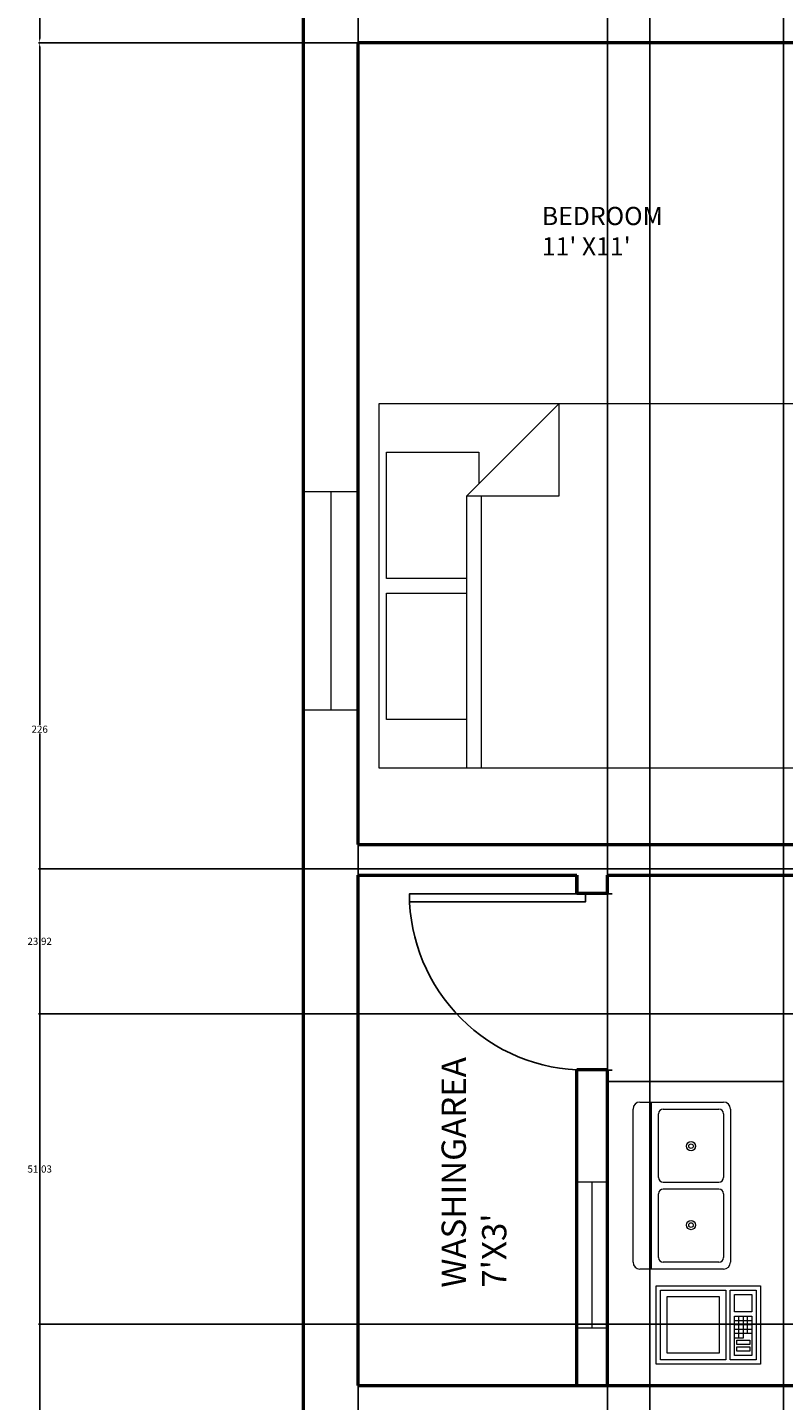
# Model space of a CAD drawing. Units: inches. Extents: x 3506 to 3958, y 1553 to 2506.
# Tile 9 of 16: x 3506 to 3631, y 2003 to 2229. Entities that reach past the tile are written whole.
import ezdxf

# ---------------------------------------------------------------- set-up
doc = ezdxf.new("R2010")
doc.units = ezdxf.units.IN
doc.header["$MEASUREMENT"] = 0
for name, color, linetype, lineweight in [('A-ANNO-DIMS', 2, 'Continuous', 18), ('A-AREA-IDEN', 7, 'Continuous', 18), ('A-FLOR-CASE', 7, 'Continuous', 25), ('A-WALL', 7, 'Continuous', 50), ('doors', 40, 'Continuous', 25), ('furniture', 120, 'Continuous', 18), ('kitchen', 181, 'Continuous', 18), ('window', 30, 'Continuous', 20)]:
    doc.layers.add(name, color=color, linetype=linetype, lineweight=lineweight)
doc.layers.add('A-WALL-PATT', color=251, linetype='Continuous', lineweight=13, true_color=0x636466)
doc.styles.get("Standard").update_dxf_attribs({"font": 'arial.ttf'})
doc.dimstyles.get("Standard").update_dxf_attribs({"dimtxt": 1.18, "dimasz": 0.68, "dimexe": 0.18, "dimexo": 0.0625, "dimgap": 0.09, "dimtad": 0, "dimtih": 1, "dimtoh": 1, "dimdec": 1, "dimzin": 0, "dimdsep": 46, "dimlunit": 3, "dimtxsty": 'Standard', "dimcen": 0.09, "dimadec": 0, "dimazin": 0, "dimtfac": 1, "dimtdec": 1, "dimtofl": 0, "dimtmove": 0, "dimatfit": 3, "dimfxl": 1, "dimtolj": 1, "dimtzin": 0, "dimarcsym": 0})

# ---------------------------------------------------------------- blocks, each defined once
blk = doc.blocks.new('*U12')
for p, q in [((0, 0), (0, 6)), ((40, 0), (40, 6))]:
    blk.add_line(p, q)
blk.add_lwpolyline([(0, 0), (0, -40), (1.75, -40), (1.75, 0)], close=True)
blk.add_arc((0, 0), 40, 270, 0)
blk = doc.blocks.new('Bed - Queen')
for p, q in [((0, -80.00003), (0, 0)), ((0, 0), (59.99999, 0)), ((59.99999, 0), (59.99999, -80.00003)), ((7.99999, -1.2), (28.79998, -1.2)), ((7.99999, -14.4), (7.99999, -1.2)), ((28.79998, -1.2), (28.79998, -14.4)), ((31.19999, -1.2), (51.99999, -1.2)), ((31.19999, -14.4), (31.19999, -1.2)), ((51.99999, -1.2), (51.99999, -16.4)), ((0, -14.4), (44.8, -14.4)), ((59.99999, -29.6), (44.8, -14.4)), ((44.8, -14.4), (44.8, -29.6)), ((44.8, -16.8), (0, -16.8)), ((51.99999, -16.4), (46.79936, -16.4)), ((44.8, -29.6), (59.99999, -29.6)), ((59.99999, -80.00003), (0, -80.00003))]:
    blk.add_line(p, q)
blk = doc.blocks.new('Microwave')
for p, q in [((18, 10), (22, 10)), ((19, 7), (19, 11)), ((20, 11), (20, 7)), ((21, 7), (21, 11)), ((22, 9), (18, 9)), ((18, 8), (22, 8)), ((22, 7), (18, 7)), ((19, 6), (19, 7)), ((20, 7), (20, 6)), ((20, 6), (18, 6))]:
    blk.add_line(p, q)
for points in [[(0, 0), (0, 18), (24, 18), (24, 0)], [(1, 1), (1, 17), (16, 17), (16, 1)], [(17, 1), (17, 17), (23, 17), (23, 1)], [(18, 12), (18, 16), (22, 16), (22, 12)], [(2.5, 2.5), (2.5, 15.5), (14.5, 15.5), (14.5, 2.5)], [(18, 2), (18, 11), (22, 11), (22, 2)], [(18.5, 4.5), (18.5, 5.5), (21.5, 5.5), (21.5, 4.5)], [(18.5, 3), (18.5, 4), (21.5, 4), (21.5, 3)]]:
    blk.add_lwpolyline(points, close=True)
blk = doc.blocks.new('Sink-double - 36 in top')
for p, q in [((-18, -4), (18, -4)), ((-0.75, -18.5), (-0.75, -6.5)), ((0.75, -6.5), (0.75, -18.5))]:
    blk.add_line(p, q)
for points in [[(-16.5, 0), (16.5, 0)], [(-18, -19.5), (-18, -1.5)], [(18, -1.5), (18, -19.5)], [(-15.5, -5.5), (-1.75, -5.5)], [(1.75, -5.5), (15.5, -5.5)], [(-16.5, -18.5), (-16.5, -6.5)], [(16.5, -6.5), (16.5, -18.5)], [(-1.75, -19.5), (-15.5, -19.5)], [(15.5, -19.5), (1.75, -19.5)], [(16.5, -21), (-16.5, -21)]]:
    blk.add_lwpolyline(points)
for centre, radius in [((-8.5, -12.5), 1), ((8.5, -12.5), 1), ((-8.5, -12.5), 0.5), ((8.5, -12.5), 0.5)]:
    blk.add_circle(centre, radius)
for centre, radius, start, end in [((-16.5, -1.5), 1.5, 90, 180), ((16.5, -1.5), 1.5, 0, 90), ((-15.5, -6.5), 1, 90, 180), ((-1.75, -6.5), 1, 0, 90), ((1.75, -6.5), 1, 90, 180), ((15.5, -6.5), 1, 0, 90), ((-16.5, -19.5), 1.5, 180, 270), ((-15.5, -18.5), 1, 180, 270), ((-1.75, -18.5), 1, 270, 0), ((1.75, -18.5), 1, 180, 270), ((15.5, -18.5), 1, 270, 0), ((16.5, -19.5), 1.5, 270, 0)]:
    blk.add_arc(centre, radius, start, end)
blk = doc.blocks.new('WIN-24IN-5IN-PARTITION')
for p, q in [((5, 24), (0, 24)), ((0, 24), (0, 0)), ((2.5, 0), (2.5, 24)), ((5, 0), (5, 24)), ((0, 0), (5, 0)), ((0, 0), (2.5, 0))]:
    blk.add_line(p, q)
blk = doc.blocks.new('*D43')
at = {"layer": 'A-ANNO-DIMS', "color": 0, "lineweight": -2, "transparency": 16777216}
for p, q in [((3560.67, 2226.39), (3508.1, 2226.39)), ((3508.28, 2225.71), (3508.28, 2114.09)), ((3508.28, 2001.07), (3508.28, 2112.7)), ((3560.67, 2000.39), (3508.1, 2000.39))]:
    blk.add_line(p, q, dxfattribs=at)
at = {"layer": 'A-ANNO-DIMS', "color": 0, "transparency": 16777216}
for points in [[(3508.17, 2225.71), (3508.39, 2225.71), (3508.28, 2226.39)], [(3508.17, 2001.07), (3508.39, 2001.07), (3508.28, 2000.39)]]:
    blk.add_solid(points, dxfattribs=at)
at = {"layer": 'Defpoints', "color": 0, "transparency": 16777216}
for p in [(3508.28, 2226.39), (3560.73, 2226.39), (3560.73, 2000.39)]:
    blk.add_point(p, dxfattribs=at)
at = {"layer": 'A-ANNO-DIMS', "color": 0, "transparency": 16777216, "insert": (3508.28, 2113.39), "char_height": 1.18, "attachment_point": 5}
blk.add_mtext('\\A1;226', dxfattribs=at)
blk = doc.blocks.new('*D44')
at = {"layer": 'A-ANNO-DIMS', "color": 0, "lineweight": -2, "transparency": 16777216}
for p, q in [((3911.67, 2461.39), (3508.1, 2461.39)), ((3508.28, 2460.71), (3508.28, 2344.59)), ((3508.28, 2227.07), (3508.28, 2343.2)), ((3560.67, 2226.39), (3508.1, 2226.39))]:
    blk.add_line(p, q, dxfattribs=at)
at = {"layer": 'A-ANNO-DIMS', "color": 0, "transparency": 16777216}
for points in [[(3508.17, 2460.71), (3508.39, 2460.71), (3508.28, 2461.39)], [(3508.17, 2227.07), (3508.39, 2227.07), (3508.28, 2226.39)]]:
    blk.add_solid(points, dxfattribs=at)
at = {"layer": 'Defpoints', "color": 0, "transparency": 16777216}
for p in [(3508.28, 2461.39), (3911.73, 2461.39), (3560.73, 2226.39)]:
    blk.add_point(p, dxfattribs=at)
at = {"layer": 'A-ANNO-DIMS', "color": 0, "transparency": 16777216, "insert": (3508.28, 2343.89), "char_height": 1.18, "attachment_point": 5}
blk.add_mtext('\\A1;235', dxfattribs=at)
blk = doc.blocks.new('*D50')
at = {"layer": 'A-ANNO-DIMS', "color": 0, "lineweight": -2, "transparency": 16777216}
for p, q in [((3608.73, 1606.46), (3608.73, 2505.02)), ((3609.41, 2504.84), (3672.39, 2504.84)), ((3738.05, 2504.84), (3675.07, 2504.84)), ((3738.73, 1606.46), (3738.73, 2505.02))]:
    blk.add_line(p, q, dxfattribs=at)
at = {"layer": 'A-ANNO-DIMS', "color": 0, "transparency": 16777216}
for points in [[(3609.41, 2504.96), (3609.41, 2504.73), (3608.73, 2504.84)], [(3738.05, 2504.96), (3738.05, 2504.73), (3738.73, 2504.84)]]:
    blk.add_solid(points, dxfattribs=at)
at = {"layer": 'Defpoints', "color": 0, "transparency": 16777216}
for p in [(3738.73, 2504.84), (3608.73, 1606.39), (3738.73, 1606.39)]:
    blk.add_point(p, dxfattribs=at)
at = {"layer": 'A-ANNO-DIMS', "color": 0, "transparency": 16777216, "insert": (3673.73, 2504.84), "char_height": 1.18, "attachment_point": 5}
blk.add_mtext('\\A1;130', dxfattribs=at)
blk = doc.blocks.new('*D52')
at = {"layer": 'A-ANNO-DIMS', "color": 0, "lineweight": -2, "transparency": 16777216}
for p, q in [((3560.73, 1606.46), (3560.73, 2505.02)), ((3561.41, 2504.84), (3583.77, 2504.84)), ((3608.05, 2504.84), (3585.69, 2504.84)), ((3608.73, 1606.46), (3608.73, 2505.02))]:
    blk.add_line(p, q, dxfattribs=at)
at = {"layer": 'A-ANNO-DIMS', "color": 0, "transparency": 16777216}
for points in [[(3561.41, 2504.96), (3561.41, 2504.73), (3560.73, 2504.84)], [(3608.05, 2504.96), (3608.05, 2504.73), (3608.73, 2504.84)]]:
    blk.add_solid(points, dxfattribs=at)
at = {"layer": 'Defpoints', "color": 0, "transparency": 16777216}
for p in [(3608.73, 2504.84), (3560.73, 1606.39), (3608.73, 1606.39)]:
    blk.add_point(p, dxfattribs=at)
at = {"layer": 'A-ANNO-DIMS', "color": 0, "transparency": 16777216, "insert": (3584.73, 2504.84), "char_height": 1.18, "attachment_point": 5}
blk.add_mtext('\\A1;48', dxfattribs=at)
blk = doc.blocks.new('*D60')
at = {"layer": 'A-ANNO-DIMS', "color": 0, "lineweight": -2, "transparency": 16777216}
for p, q in [((3860.67, 2066.52), (3508.1, 2066.52)), ((3508.28, 2065.84), (3508.28, 2041.7)), ((3508.28, 2016.17), (3508.28, 2040.31)), ((3860.67, 2015.49), (3508.1, 2015.49))]:
    blk.add_line(p, q, dxfattribs=at)
at = {"layer": 'A-ANNO-DIMS', "color": 0, "transparency": 16777216}
for points in [[(3508.17, 2065.84), (3508.39, 2065.84), (3508.28, 2066.52)], [(3508.17, 2016.17), (3508.39, 2016.17), (3508.28, 2015.49)]]:
    blk.add_solid(points, dxfattribs=at)
at = {"layer": 'Defpoints', "color": 0, "transparency": 16777216}
for p in [(3860.73, 2066.52), (3508.28, 2015.49), (3860.73, 2015.49)]:
    blk.add_point(p, dxfattribs=at)
at = {"layer": 'A-ANNO-DIMS', "color": 0, "transparency": 16777216, "insert": (3508.28, 2041), "char_height": 1.18, "attachment_point": 5}
blk.add_mtext('\\A1;51.03', dxfattribs=at)
blk = doc.blocks.new('*D61')
at = {"layer": 'A-ANNO-DIMS', "color": 0, "lineweight": -2, "transparency": 16777216}
for p, q in [((3860.67, 2090.43), (3508.1, 2090.43)), ((3508.28, 2089.75), (3508.28, 2079.17)), ((3508.28, 2067.2), (3508.28, 2077.78)), ((3860.67, 2066.52), (3508.1, 2066.52))]:
    blk.add_line(p, q, dxfattribs=at)
at = {"layer": 'A-ANNO-DIMS', "color": 0, "transparency": 16777216}
for points in [[(3508.17, 2089.75), (3508.39, 2089.75), (3508.28, 2090.43)], [(3508.17, 2067.2), (3508.39, 2067.2), (3508.28, 2066.52)]]:
    blk.add_solid(points, dxfattribs=at)
at = {"layer": 'Defpoints', "color": 0, "transparency": 16777216}
for p in [(3860.73, 2090.43), (3508.28, 2066.52), (3860.73, 2066.52)]:
    blk.add_point(p, dxfattribs=at)
at = {"layer": 'A-ANNO-DIMS', "color": 0, "transparency": 16777216, "insert": (3508.28, 2078.48), "char_height": 1.18, "attachment_point": 5}
blk.add_mtext('\\A1;23.92', dxfattribs=at)
blk = doc.blocks.new('*D68')
at = {"layer": 'A-ANNO-DIMS', "color": 0, "lineweight": -2, "transparency": 16777216}
for p, q in [((3630.73, 2260.33), (3630.73, 1553.76)), ((3601.73, 2231.33), (3601.73, 1553.76)), ((3602.41, 1553.94), (3615.28, 1553.94)), ((3630.05, 1553.94), (3617.18, 1553.94))]:
    blk.add_line(p, q, dxfattribs=at)
at = {"layer": 'A-ANNO-DIMS', "color": 0, "transparency": 16777216}
for points in [[(3602.41, 1554.06), (3602.41, 1553.83), (3601.73, 1553.94)], [(3630.05, 1554.06), (3630.05, 1553.83), (3630.73, 1553.94)]]:
    blk.add_solid(points, dxfattribs=at)
at = {"layer": 'Defpoints', "color": 0, "transparency": 16777216}
for p in [(3630.73, 2260.39), (3601.73, 2231.39), (3630.73, 1553.94)]:
    blk.add_point(p, dxfattribs=at)
at = {"layer": 'A-ANNO-DIMS', "color": 0, "transparency": 16777216, "insert": (3616.23, 1553.94), "char_height": 1.18, "attachment_point": 5}
blk.add_mtext('\\A1;29', dxfattribs=at)

msp = doc.modelspace()

# ---------------------------------------------------------------- hatches: boundary and pattern name
at = {"layer": 'A-WALL-PATT'}
h = msp.add_hatch(dxfattribs=at)
h.set_pattern_fill('ANSI31', color=256)
h.paths.add_polyline_path([(3911.7302, 2461.3942), (3551.7302, 2461.3942), (3551.7302, 2152.516), (3560.7302, 2152.516), (3560.7302, 2116.516), (3551.7302, 2116.516), (3551.7302, 1920.5711), (3556.2302, 1920.5711), (3560.7302, 1920.5711), (3560.7302, 2000.3942), (3692.7302, 2000.3942), (3692.7302, 1997.3942), (3697.7302, 1997.3942), (3697.7302, 2000.3942), (3771.7302, 2000.3942), (3771.7302, 1997.3942), (3776.7302, 1997.3942), (3776.7302, 1997.7206), (3778.5802, 1997.7206), (3807.5802, 1997.7206), (3807.5802, 1996.4519), (3778.5802, 1996.4519), (3778.5802, 1997.7206), (3776.7302, 1997.7206), (3776.7302, 1997.3942), (3771.7302, 1997.3942), (3771.7302, 2000.3942), (3697.7302, 2000.3942), (3697.7302, 1997.3942), (3692.7302, 1997.3942), (3689.8302, 1997.3942), (3689.8302, 1995.8192), (3653.8302, 1995.8192), (3653.8302, 1997.3942), (3689.8302, 1997.3942), (3692.7302, 1997.3942), (3692.7302, 2000.3942), (3560.7302, 2000.3942), (3560.7302, 1920.5711), (3551.7302, 1920.5711), (3551.7302, 1884.5711), (3551.7302, 1597.3942), (3911.7302, 1597.3942)], flags=17)
h.paths.add_polyline_path([(3596.7302, 2005.3942), (3596.7302, 2057.3035, -0.38730371), (3569.1778, 2085), (3569.15, 2085), (3569.15, 2086.2688), (3598.15, 2086.2688), (3598.15, 2085), (3569.1778, 2085, 0.38730371), (3596.7302, 2057.3035), (3596.7302, 2057.3942), (3601.7302, 2057.3942), (3601.7302, 2055.3942), (3630.7302, 2055.3942), (3630.7302, 2034.3942), (3694.7302, 2034.3942), (3694.7302, 2053.3942), (3699.7302, 2053.3942), (3699.7302, 2005.3942), (3860.7302, 2005.3942), (3860.7302, 2173.3942), (3771.7302, 2173.3942), (3771.7302, 2194.3942), (3776.7302, 2194.3942), (3776.7302, 2178.3942), (3860.7302, 2178.3942), (3860.7302, 2231.3942), (3601.7302, 2231.3942), (3601.7302, 2241.426), (3596.7302, 2241.426), (3596.7302, 2231.3942), (3560.7302, 2231.3942), (3560.7302, 2315.3942), (3596.7302, 2315.3942), (3596.7302, 2312.3942), (3601.7302, 2312.3942), (3601.7302, 2315.3942), (3697.7302, 2315.3942), (3697.7302, 2413.3942), (3692.7302, 2413.3942), (3692.7302, 2320.3942), (3560.7302, 2320.3942), (3560.7302, 2452.3942), (3692.7302, 2452.3942), (3692.7302, 2449.3942), (3697.7302, 2449.3942), (3697.7302, 2452.3942), (3771.7302, 2452.3942), (3771.7302, 2449.3942), (3776.7302, 2449.3942), (3776.7302, 2452.3942), (3860.7302, 2452.3942), (3860.7302, 2437.2075), (3865.2302, 2437.2075), (3865.2302, 2413.2075), (3860.7302, 2413.2075), (3860.7302, 2367.6976), (3865.2302, 2367.6976), (3869.7302, 2367.6976), (3869.7302, 2319.6976), (3860.7302, 2319.6976), (3860.7302, 2211.6248), (3869.7302, 2211.6248), (3869.7302, 2187.6248), (3860.7302, 2187.6248), (3860.7302, 2138.4346), (3865.2302, 2138.4346), (3869.7302, 2138.4346), (3869.7302, 2090.4346), (3860.7302, 2090.4346), (3860.7302, 1985.8449), (3869.7302, 1985.8449), (3869.7302, 1961.8449), (3860.7302, 1961.8449), (3860.7302, 1897.0756), (3865.2302, 1897.0756), (3869.7302, 1897.0756), (3869.7302, 1849.0756), (3860.7302, 1849.0756), (3860.7302, 1847.8112), (3860.7302, 1779.3942), (3596.7302, 1779.3942), (3596.7302, 1831.3942), (3601.7302, 1831.3942), (3601.7302, 1828.3942), (3630.7302, 1828.3942), (3630.7302, 1808.3942), (3691.7302, 1808.3942), (3691.7302, 1815.3942), (3696.7302, 1815.3942), (3696.7302, 1779.3942), (3860.7302, 1779.3942), (3860.7302, 1947.3942), (3771.7302, 1947.3942), (3771.7302, 1968.3942), (3776.7302, 1968.3942), (3776.7302, 1952.3942), (3860.7302, 1952.3942), (3860.7302, 2005.3942)], flags=0)
h.paths.add_polyline_path([(3596.7302, 2038.8546), (3601.7302, 2038.8546), (3601.7302, 2014.8546), (3596.7302, 2014.8546)], flags=0)
h.paths.add_polyline_path([(3564.1688, 2107), (3564.1688, 2167), (3644.1688, 2167), (3644.1688, 2107)], flags=0)
h.paths.add_polyline_path([(3607.0972, 2052.0208), (3620.8472, 2052.0208, -0.41421356), (3621.9931, 2050.875), (3621.9931, 2025.6667, -0.41421356), (3620.8472, 2024.5208), (3607.0972, 2024.5208, -0.41421356), (3605.9514, 2025.6667), (3605.9514, 2050.875, -0.41421356)], flags=0)
h.paths.add_polyline_path([(3578.5688, 2115), (3565.3688, 2115), (3565.3688, 2135.8), (3578.5688, 2135.8), (3578.5688, 2138.2), (3565.3688, 2138.2), (3565.3688, 2159), (3580.5688, 2159), (3580.5688, 2153.8), (3593.7688, 2167), (3593.7688, 2151.8), (3578.5688, 2151.8)], flags=0)
h.paths.add_polyline_path([(3610.9167, 2050.875), (3620.0833, 2050.875, -0.41421356), (3620.8472, 2050.1111), (3620.8472, 2039.6076, -0.41421356), (3620.0833, 2038.8438), (3610.9167, 2038.8438, -0.41421356), (3610.1528, 2039.6076), (3610.1528, 2050.1111, -0.41421356)], flags=0)
h.paths.add_polyline_path([(3610.9167, 2037.6979), (3620.0833, 2037.6979, -0.41421356), (3620.8472, 2036.934), (3620.8472, 2026.4306, -0.41421356), (3620.0833, 2025.6667), (3610.9167, 2025.6667, -0.41421356), (3610.1528, 2026.4306), (3610.1528, 2036.934, -0.41421356)], flags=0)
h.paths.add_polyline_path([(3616.2639, 2044.7639, -1), (3614.7361, 2044.7639, -1)], flags=0)
h.paths.add_polyline_path([(3615.8819, 2044.7639, -1), (3615.1181, 2044.7639, -1)], flags=0)
h.paths.add_polyline_path([(3616.2639, 2031.7778, -1), (3614.7361, 2031.7778, -1)], flags=0)
h.paths.add_polyline_path([(3615.8819, 2031.7778, -1), (3615.1181, 2031.7778, -1)], flags=0)
h.paths.add_polyline_path([(3609.7539, 2021.7868), (3626.9586, 2021.7868), (3626.9586, 2008.8833), (3609.7539, 2008.8833)], flags=0)
h.paths.add_polyline_path([(3610.4708, 2021.07), (3621.2237, 2021.07), (3621.2237, 2009.6002), (3610.4708, 2009.6002)], flags=0)
h.paths.add_polyline_path([(3611.5461, 2019.9947), (3620.1484, 2019.9947), (3620.1484, 2010.6755), (3611.5461, 2010.6755)], flags=0)
h.paths.add_polyline_path([(3621.9405, 2021.07), (3626.2417, 2021.07), (3626.2417, 2009.6002), (3621.9405, 2009.6002)], flags=0)
h.paths.add_polyline_path([(3622.6574, 2020.3531), (3625.5248, 2020.3531), (3625.5248, 2017.4857), (3622.6574, 2017.4857)], flags=0)
h.paths.add_polyline_path([(3622.6574, 2016.7688), (3625.5248, 2016.7688), (3625.5248, 2010.317), (3622.6574, 2010.317)], flags=0)
h.paths.add_polyline_path([(3624.808, 2016.0519), (3624.808, 2013.9013), (3624.0911, 2013.9013), (3624.0911, 2013.1845), (3623.3743, 2013.1845), (3623.3743, 2013.9013), (3623.3743, 2016.0519)], flags=0)
h.paths.add_polyline_path([(3623.0158, 2012.8261), (3625.1664, 2012.8261), (3625.1664, 2012.1092), (3623.0158, 2012.1092)], flags=0)
h.paths.add_polyline_path([(3623.0158, 2011.7508), (3625.1664, 2011.7508), (3625.1664, 2011.0339), (3623.0158, 2011.0339)], flags=0)
h.paths.add_polyline_path([(3650.0591, 2031.8202), (3674.0368, 2031.8202), (3674.0368, 2012.638), (3669.2413, 2012.638), (3669.2413, 2011.8388), (3672.4383, 2011.8388), (3672.4383, 2011.0395), (3651.6576, 2011.0395), (3651.6576, 2011.8388), (3654.8546, 2011.8388), (3654.8546, 2012.638), (3650.0591, 2012.638)], flags=0)
h.paths.add_polyline_path([(3658.0517, 2024.6269, -1), (3651.6576, 2024.6269, -1)], flags=0)
h.paths.add_polyline_path([(3657.2524, 2024.6269, -1), (3652.4569, 2024.6269, -1)], flags=0)
h.paths.add_polyline_path([(3656.4532, 2024.6269, -1), (3653.2561, 2024.6269, -1)], flags=0)
h.paths.add_polyline_path([(3655.6539, 2024.6269, -1), (3654.0554, 2024.6269, -1)], flags=0)
h.paths.add_polyline_path([(3657.2524, 2017.4336, -1), (3652.4569, 2017.4336, -1)], flags=0)
h.paths.add_polyline_path([(3656.4532, 2017.4336, -1), (3653.2561, 2017.4336, -1)], flags=0)
h.paths.add_polyline_path([(3655.6539, 2017.4336, -1), (3654.0554, 2017.4336, -1)], flags=0)
h.paths.add_polyline_path([(3659.6502, 2027.8239), (3664.4457, 2027.8239), (3664.4457, 2015.0358), (3659.6502, 2015.0358)], flags=0)
h.paths.add_polyline_path([(3663.6465, 2027.0247), (3663.6465, 2015.8351), (3660.4494, 2015.8351), (3660.4494, 2027.0247)], flags=0)
h.paths.add_polyline_path([(3562.6688, 1945.5), (3642.6688, 1945.5), (3642.6688, 1885.5), (3562.6688, 1885.5)], flags=0)
h.paths.add_polyline_path([(3671.6391, 2024.6269, -1), (3666.8435, 2024.6269, -1)], flags=0)
h.paths.add_polyline_path([(3670.8398, 2024.6269, -1), (3667.6428, 2024.6269, -1)], flags=0)
h.paths.add_polyline_path([(3672.4383, 2017.4336, -1), (3666.0443, 2017.4336, -1)], flags=0)
h.paths.add_polyline_path([(3670.0405, 2024.6269, -1), (3668.442, 2024.6269, -1)], flags=0)
h.paths.add_polyline_path([(3671.6391, 2017.4336, -1), (3666.8435, 2017.4336, -1)], flags=0)
h.paths.add_polyline_path([(3670.8398, 2017.4336, -1), (3667.6428, 2017.4336, -1)], flags=0)
h.paths.add_polyline_path([(3592.2688, 1945.5), (3592.2688, 1930.3), (3577.0688, 1930.3), (3577.0688, 1893.5), (3563.8688, 1893.5), (3563.8688, 1914.3), (3577.0688, 1914.3), (3577.0688, 1916.7), (3563.8688, 1916.7), (3563.8688, 1937.5), (3579.0688, 1937.5), (3579.0688, 1932.3)], flags=0)
h.paths.add_polyline_path([(3670.0405, 2017.4336, -1), (3668.442, 2017.4336, -1)], flags=0)
h.paths.add_polyline_path([(3596.7302, 2283.3942), (3601.7302, 2283.3942), (3601.7302, 2265.426), (3599.2302, 2265.426), (3599.2302, 2241.426), (3596.7302, 2241.426), (3596.7302, 2265.426)], flags=0)
h.paths.add_polyline_path([(3596.7302, 1810.7006), (3601.7302, 1810.7006), (3601.7302, 1786.7006), (3596.7302, 1786.7006)], flags=0)
h.paths.add_polyline_path([(3560.7302, 1770.3942), (3738.7302, 1770.3942), (3738.7302, 1746.3942), (3738.7302, 1722.3942), (3748.7302, 1722.3942), (3748.7302, 1674.3942), (3560.7302, 1674.3942)], flags=0)
h.paths.add_polyline_path([(3728.7302, 1746.3942), (3728.7302, 1756.0642), (3738.7302, 1746.3942), (3728.7302, 1738.1582), (3728.7302, 1698.3942), (3591.2519, 1698.3942), (3591.2519, 1746.3942)], flags=0)
h.paths.add_polyline_path([(3771.7302, 2399.3942), (3771.7302, 2420.3942), (3776.7302, 2420.3942), (3776.7302, 2404.3942), (3776.7302, 2399.3942)], flags=0)
h.paths.add_polyline_path([(3911.7302, 2461.3942), (3551.7302, 2461.3942), (3551.7302, 2152.516), (3560.7302, 2152.516), (3560.7302, 2116.516), (3551.7302, 2116.516), (3551.7302, 1920.5711), (3560.7302, 1920.5711), (3560.7302, 2000.3942), (3692.7302, 2000.3942), (3692.7302, 1997.3942), (3697.7302, 1997.3942), (3697.7302, 2000.3942), (3771.7302, 2000.3942), (3771.7302, 1997.3942), (3776.7302, 1997.3942), (3776.7302, 1997.7206), (3778.5802, 1997.7206), (3807.5802, 1997.7206), (3807.5802, 1996.4519), (3778.5802, 1996.4519), (3778.5802, 1997.7206), (3776.7302, 1997.7206), (3776.7302, 1997.3942), (3771.7302, 1997.3942), (3771.7302, 2000.3942), (3697.7302, 2000.3942), (3697.7302, 1997.3942), (3692.7302, 1997.3942), (3689.8302, 1997.3942), (3689.8302, 1995.8192), (3653.8302, 1995.8192), (3653.8302, 1997.3942), (3689.8302, 1997.3942), (3692.7302, 1997.3942), (3692.7302, 2000.3942), (3560.7302, 2000.3942), (3560.7302, 1920.5711), (3551.7302, 1920.5711), (3551.7302, 1597.3942), (3911.7302, 1597.3942)], flags=17)

# ---------------------------------------------------------------- linework, layer by layer
at = {"layer": 'A-FLOR-CASE'}
msp.add_line((3601.7302, 2055.3942), (3630.7302, 2055.3942), dxfattribs=at)
at = {"layer": 'A-WALL'}
for p, q in [((3560.7302, 2226.3942), (3692.7302, 2226.3942)), ((3560.7302, 2094.3942), (3560.7302, 2226.3942)), ((3560.7302, 2094.3942), (3692.7302, 2094.3942)), ((3560.7302, 2089.3942), (3596.7302, 2089.3942)), ((3560.7302, 2005.3942), (3560.7302, 2089.3942)), ((3596.7302, 2089.3942), (3596.7302, 2086.3942)), ((3596.7302, 2086.3942), (3596.7302, 2089.3942)), ((3601.7302, 2086.3942), (3601.7302, 2089.3942)), ((3601.7302, 2089.3942), (3697.7302, 2089.3942)), ((3596.7302, 2086.3942), (3601.7302, 2086.3942)), ((3596.7302, 2057.3942), (3601.7302, 2057.3942)), ((3596.7302, 2005.3942), (3596.7302, 2057.3942)), ((3596.7302, 2057.3942), (3601.7302, 2057.3942)), ((3596.7302, 2057.3942), (3601.7302, 2057.3942)), ((3601.7302, 2005.3942), (3601.7302, 2057.3942)), ((3560.7302, 2005.3942), (3860.7302, 2005.3942))]:
    msp.add_line(p, q, dxfattribs=at)
msp.add_lwpolyline([(3551.7302, 2461.3942), (3911.7302, 2461.3942), (3911.7302, 1597.3942), (3551.7302, 1597.3942)], close=True, dxfattribs=at)
at = {"layer": 'window'}
for p, q in [((3551.7302, 2152.516), (3560.7302, 2152.516)), ((3556.2302, 2152.516), (3556.2302, 2116.516)), ((3560.7302, 2152.516), (3560.7302, 2116.516)), ((3560.7302, 2116.516), (3551.7302, 2116.516))]:
    msp.add_line(p, q, dxfattribs=at)

# ---------------------------------------------------------------- block references
at = {"layer": 'doors', "xscale": 0.725, "yscale": 0.725, "zscale": 0.725, "rotation": 270}
msp.add_blockref('*U12', (3598.15, 2086.2688), dxfattribs=at)
at = {"layer": 'furniture', "rotation": 90}
msp.add_blockref('Bed - Queen', (3564.1688, 2107), dxfattribs=at)
at = {"layer": 'kitchen', "xscale": 0.763888888888889, "yscale": 0.763888888888889, "zscale": 0.763888888888889, "rotation": 90}
msp.add_blockref('Sink-double - 36 in top', (3605.9514, 2038.2708), dxfattribs=at)
at = {"layer": 'kitchen', "xscale": 0.7168604389202189, "yscale": 0.7168604389202189, "zscale": 0.7168604389202189}
msp.add_blockref('Microwave', (3609.7539, 2008.8833), dxfattribs=at)
at = {"layer": 'window'}
msp.add_blockref('WIN-24IN-5IN-PARTITION', (3596.73, 2014.855), dxfattribs=at)

# ---------------------------------------------------------------- texts
at = {"layer": 'A-AREA-IDEN', "insert": (3590.9424, 2199.3653), "char_height": 3, "attachment_point": 1}
msp.add_mtext_dynamic_manual_height_columns("BEDROOM\\P11' X11'", width=46.119714, gutter_width=1, heights=[0], dxfattribs=at)
at = {"layer": 'A-AREA-IDEN', "insert": (3574.4345, 2021.4695), "char_height": 4, "attachment_point": 1, "rotation": 90}
msp.add_mtext_dynamic_manual_height_columns("WASHINGAREA\\P 7'X3'", width=7.450055, gutter_width=1, heights=[0], dxfattribs=at)

# ---------------------------------------------------------------- dimensions: what is measured, and where the dimension line sits
at = {"layer": 'A-ANNO-DIMS'}
for base, p1, p2, picture, middle in [((3608.7302, 2504.8442), (3560.7302, 1606.3942), (3608.7302, 1606.3942), '*D52', (3584.7302, 2504.8442)), ((3738.7302, 2504.8442), (3608.7302, 1606.3942), (3738.7302, 1606.3942), '*D50', (3673.7302, 2504.8442)), ((3630.7302, 1553.9442), (3601.7302, 2231.3942), (3630.7302, 2260.3942), '*D68', (3616.2302, 1553.9442))]:
    dim = msp.add_linear_dim(base=base, p1=p1, p2=p2, dimstyle='Standard', override={"dimdec": 0, "dimlfac": 1, "dimrnd": 0, "dimzin": 0, "dimdsep": 46, "dimlunit": 2}, dxfattribs=at)
    dim.commit()
    dim.dimension.update_dxf_attribs({"geometry": picture, "text_midpoint": middle})
for base, p1, p2, override, picture, middle in [((3508.2802, 2461.3942), (3560.7302, 2226.3942), (3911.7302, 2461.3942), {"dimdec": 0, "dimlfac": 1, "dimrnd": 0, "dimzin": 0, "dimdsep": 46, "dimlunit": 2}, '*D44', (3508.2802, 2343.8942)), ((3508.2802, 2226.3942), (3560.7302, 2000.3942), (3560.7302, 2226.3942), {"dimdec": 0, "dimlfac": 1, "dimrnd": 0, "dimzin": 0, "dimdsep": 46, "dimlunit": 2}, '*D43', (3508.2802, 2113.3942)), ((3508.2802, 2066.516), (3860.7302, 2090.4346), (3860.7302, 2066.516), {"dimdec": 2, "dimlfac": 1, "dimrnd": 0, "dimzin": 0, "dimdsep": 46, "dimlunit": 2}, '*D61', (3508.2802, 2078.4753)), ((3508.2802, 2015.4906), (3860.7302, 2066.516), (3860.7302, 2015.4906), {"dimdec": 2, "dimlfac": 1, "dimrnd": 0, "dimzin": 0, "dimdsep": 46, "dimlunit": 2}, '*D60', (3508.2802, 2041.0033))]:
    dim = msp.add_linear_dim(base=base, p1=p1, p2=p2, angle=90, dimstyle='Standard', override=override, dxfattribs=at)
    dim.commit()
    dim.dimension.update_dxf_attribs({"geometry": picture, "text_midpoint": middle})

doc.saveas('drawing.dxf')
